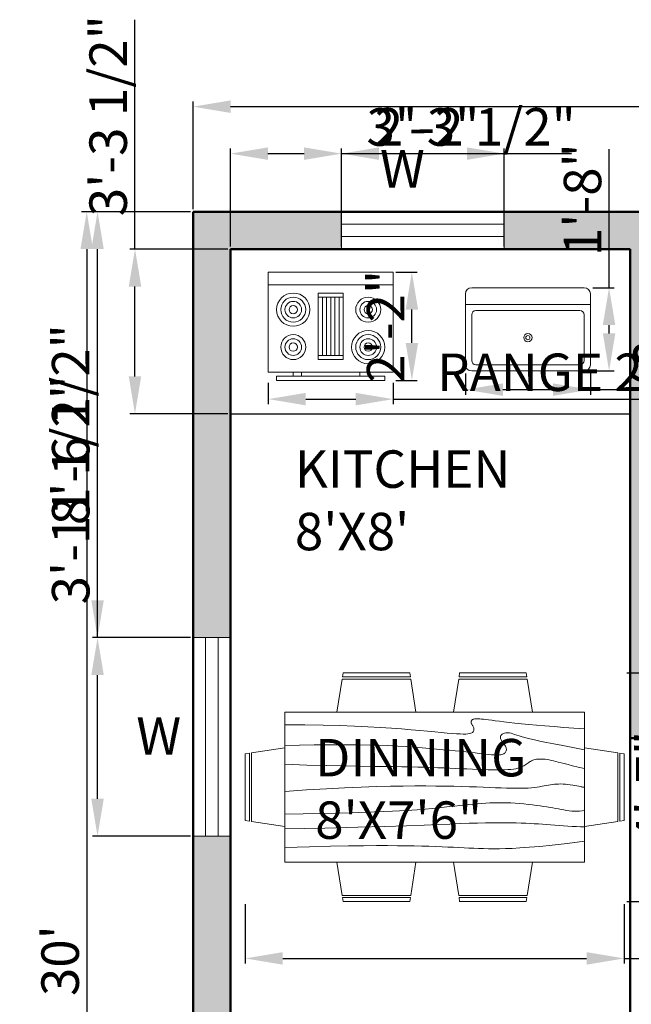
# Model space of a CAD drawing. Units: inches. Extents: x 16989 to 17950, y 7982 to 8536.
# Tile 2 of 5: x 16989 to 17136, y 8270 to 8506. Entities that reach past the tile are written whole.
import ezdxf

# ---------------------------------------------------------------- set-up
doc = ezdxf.new("R2010")
doc.units = ezdxf.units.IN
for name, color, linetype, lineweight in [('A-ANNO-DIMS', 2, 'Continuous', 18), ('A-ANNO-IDEN', 7, 'Continuous', 18), ('A-AREA-IDEN', 7, 'Continuous', 25), ('A-EQPM', 8, 'Continuous', 18), ('A-FLOR-CASE', 8, 'Continuous', 25), ('A-FLOR-FIXT', 9, 'Continuous', 18), ('A-FURN', 8, 'Continuous', 18), ('A-GLAZ', 4, 'Continuous', 18), ('A-WALL', 7, 'Continuous', 50)]:
    doc.layers.add(name, color=color, linetype=linetype, lineweight=lineweight)
doc.layers.add('A-WALL-PATT', color=177, linetype='Continuous', lineweight=13, true_color=0x293189)
doc.styles.get("Standard").update_dxf_attribs({"font": 'arial.ttf'})
doc.dimstyles.new('ISO-25', dxfattribs={"dimtxt": 9, "dimasz": 9, "dimexe": 1.25, "dimexo": 0.625, "dimtad": 1, "dimdec": 1, "dimrnd": 9, "dimlunit": 3, "dimtxsty": 'Standard', "dimcen": 2.5, "dimadec": 0, "dimazin": 0, "dimtfac": 1, "dimtdec": 1, "dimtmove": 0, "dimatfit": 3, "dimfxl": 1, "dimarcsym": 0})

# ---------------------------------------------------------------- blocks, each defined once
blk = doc.blocks.new('Range-Oven - 30 in top')
for p, q in [((0, -3), (30, -3)), ((12, -6), (18, -6)), ((13, -20), (13, -6)), ((14, -6), (14, -20)), ((15, -20), (15, -6)), ((16, -6), (16, -20)), ((17, -20), (17, -6)), ((18, -20), (12, -20)), ((6, -24), (6, -25)), ((8, -25), (8, -24)), ((22, -25), (22, -24)), ((24, -24), (24, -25))]:
    blk.add_line(p, q)
for points in [[(0, -24), (0, 0), (30, 0), (30, -24)], [(12, -21), (12, -5), (18, -5), (18, -21)], [(2, -26), (2, -25), (28, -25), (28, -26)]]:
    blk.add_lwpolyline(points, close=True)
for centre, radius in [((6, -9), 4), ((6, -9), 3), ((6, -9), 2), ((24, -9), 3), ((24, -9), 2), ((6, -9), 1), ((24, -9), 1), ((24, -18), 4), ((6, -18), 3), ((6, -18), 2), ((24, -18), 3), ((24, -18), 2), ((6, -18), 1), ((24, -18), 1)]:
    blk.add_circle(centre, radius)
blk = doc.blocks.new('Sink-single - 30 in top')
blk.add_line((-15, -3.999996), (15, -3.999996))
for points in [[(-13.5, 0), (13.5, 0)], [(-15, -18.499996), (-15, -1.5)], [(15, -1.5), (15, -18.499996)], [(-13.5, -17.499996), (-13.5, -6.499996)], [(-12.5, -5.499996), (12.5, -5.499996)], [(13.5, -6.499996), (13.5, -17.499996)], [(12.5, -18.499996), (-12.5, -18.499996)], [(13.5, -19.999996), (-13.5, -19.999996)]]:
    blk.add_lwpolyline(points)
for radius in [1, 0.5]:
    blk.add_circle((0, -11.999996), radius)
for centre, radius, start, end in [((-13.5, -1.5), 1.5, 90, 180), ((13.5, -1.5), 1.5, 0, 90), ((-12.5, -6.499996), 1, 90, 180), ((12.5, -6.499996), 1, 0, 90), ((-13.5, -18.499996), 1.5, 180, 270), ((-12.5, -17.499996), 1, 180, 270), ((12.5, -17.499996), 1, 270, 0), ((13.5, -18.499996), 1.5, 270, 0)]:
    blk.add_arc(centre, radius, start, end)
blk = doc.blocks.new('Dining Set - 36 x 72 in.')
for p, q in [((-22, 27.5), (-22.1562, 26.50042)), ((-5.8416, 26.5), (-22.1534, 26.5)), ((-22, 27.5), (-6, 27.5)), ((-5.8437, 26.49966), (-6, 27.5)), ((6, 27.5), (5.8438, 26.50042)), ((22.1584, 26.5), (5.8466, 26.5)), ((6, 27.5), (22, 27.5)), ((22.1563, 26.49966), (22, 27.5)), ((-22.2343, 26.00059), (-23.4847, 17.99762)), ((-22.2304, 26), (-5.7608, 26)), ((-4.5152, 17.99762), (-5.7655, 25.99926)), ((5.7657, 26.00059), (4.5153, 17.99762)), ((5.7696, 26), (22.2392, 26)), ((23.4848, 17.99762), (22.2345, 25.99926)), ((36, 18), (-36, 18)), ((-36, 18), (-36, -18)), ((36, -18), (36, 18)), ((-44.0006, 8.23428), (-35.9976, 9.48474)), ((44.0006, 8.23428), (35.9976, 9.48474)), ((-45.5, 8), (-44.5004, 8.15617)), ((-45.5, 8), (-45.5, -8)), ((-44.5, -8.15843), (-44.5, 8.15338)), ((-44, 8.23041), (-44, -8.23915)), ((44, 8.23041), (44, -8.23915)), ((44.5, -8.15843), (44.5, 8.15338)), ((45.5, 8), (44.5005, 8.15617)), ((45.5, 8), (45.5, -8)), ((-44.4997, -8.15631), (-45.5, -8)), ((-35.9976, -9.48476), (-43.9993, -8.2345)), ((35.9976, -9.48476), (43.9993, -8.2345)), ((44.4997, -8.15631), (45.5, -8)), ((-36, -18), (36, -18)), ((-22.2343, -26.0006), (-23.4847, -17.99762)), ((-4.5152, -17.99762), (-5.7655, -25.99928)), ((5.7657, -26.0006), (4.5153, -17.99762)), ((23.4848, -17.99762), (22.2345, -25.99928)), ((-22.2304, -26), (-5.7608, -26)), ((5.7696, -26), (22.2392, -26)), ((-22, -27.5), (-22.1562, -26.50044)), ((-5.8416, -26.5), (-22.1534, -26.5)), ((-22, -27.5), (-6, -27.5)), ((-5.8437, -26.49967), (-6, -27.5)), ((6, -27.5), (5.8438, -26.50044)), ((22.1584, -26.5), (5.8466, -26.5)), ((6, -27.5), (22, -27.5)), ((22.1563, -26.49967), (22, -27.5))]:
    blk.add_line(p, q)
for points in [[(-36, 15), (-31.1772, 14.97754), (-26.8079, 14.91406), (-22.8538, 14.81543), (-19.276, 14.6875), (-16.0362, 14.53613), (-13.0957, 14.36718), (-10.4159, 14.18652), (-7.9583, 14), (-5.6904, 13.81315), (-3.6035, 13.63021), (-1.6954, 13.45508), (0.0365, 13.29166), (1.5945, 13.14388), (2.9811, 13.01562), (4.1988, 12.9108), (5.25, 12.83333), (6.1393, 12.78613), (6.8802, 12.76823), (7.4883, 12.77767), (7.9792, 12.8125), (8.3685, 12.87077), (8.6719, 12.95052), (8.9049, 13.0498), (9.0833, 13.16666), (9.2205, 13.29899), (9.3216, 13.44401), (9.3895, 13.59879), (9.4271, 13.76041), (9.4373, 13.92594), (9.4232, 14.09245), (9.3875, 14.257), (9.3333, 14.41666), (9.2638, 14.56917), (9.1836, 14.71484), (9.0975, 14.85465), (9.0104, 14.98958), (8.9272, 15.1206), (8.8529, 15.2487), (8.7922, 15.37483), (8.75, 15.5), (8.7305, 15.62467), (8.7344, 15.74739), (8.7617, 15.86621), (8.8125, 15.97916), (8.8867, 16.08431), (8.9844, 16.17968), (9.1055, 16.26334), (9.25, 16.33333), (9.4189, 16.38802), (9.6172, 16.42708), (9.8506, 16.45052), (10.125, 16.45833), (10.4463, 16.45052), (10.8203, 16.42708), (11.2529, 16.38802), (11.75, 16.33333), (12.3184, 16.26318), (12.9694, 16.17838), (13.7151, 16.07991), (14.5677, 15.96875), (15.5395, 15.84586), (16.6426, 15.71224), (17.8893, 15.56884), (19.2917, 15.41666), (20.859, 15.25667), (22.5879, 15.08984), (24.4721, 14.91715), (26.5052, 14.73958), (28.6809, 14.5581), (30.9929, 14.3737), (33.4347, 14.18733), (36, 14)], [(-36, 10), (-28.9766, 10.14274), (-23.1725, 10.20442), (-18.4241, 10.19775), (-14.5677, 10.13541), (-11.4399, 10.03011), (-8.877, 9.89453), (-6.7154, 9.74137), (-4.7917, 9.58333), (-2.9698, 9.43082), (-1.2246, 9.28515), (0.4415, 9.14534), (2.026, 9.01041), (3.5266, 8.87939), (4.9408, 8.7513), (6.266, 8.62516), (7.5, 8.5), (8.6411, 8.37549), (9.6914, 8.2539), (10.6538, 8.13818), (11.5312, 8.03125), (12.3267, 7.93603), (13.043, 7.85547), (13.6831, 7.79248), (14.25, 7.75), (14.7471, 7.7303), (15.1797, 7.73307), (15.5537, 7.75732), (15.875, 7.80208), (16.1494, 7.86637), (16.3828, 7.94922), (16.5811, 8.04964), (16.75, 8.16666), (16.8944, 8.29915), (17.0143, 8.44531), (17.1089, 8.60319), (17.1771, 8.77083), (17.218, 8.94629), (17.2305, 9.1276), (17.2137, 9.31282), (17.1667, 9.5), (17.0895, 9.6875), (16.987, 9.875), (16.8649, 10.0625), (16.7292, 10.25), (16.5856, 10.4375), (16.4401, 10.625), (16.2985, 10.8125), (16.1667, 11), (16.05, 11.18733), (15.9518, 11.3737), (15.8752, 11.5581), (15.8229, 11.73958), (15.798, 11.91715), (15.8034, 12.08984), (15.842, 12.25667), (15.9167, 12.41666), (16.0295, 12.56836), (16.1784, 12.70833), (16.3605, 12.83268), (16.5729, 12.9375), (16.8127, 13.01888), (17.0768, 13.07291), (17.3625, 13.0957), (17.6667, 13.08333), (17.9894, 13.03312), (18.3418, 12.94726), (18.7382, 12.82918), (19.1927, 12.68229), (19.7195, 12.51001), (20.3327, 12.31575), (21.0465, 12.10294), (21.875, 11.875), (22.8357, 11.63354), (23.959, 11.37304), (25.2786, 11.08618), (26.8282, 10.76562), (28.6414, 10.40405), (30.752, 9.99414), (33.1936, 9.52856), (36, 9)], [(-36, 5.5), (-30.7157, 5.3348), (-26.069, 5.20963), (-21.9946, 5.11767), (-18.4271, 5.05208), (-15.3009, 5.00602), (-12.5508, 4.97265), (-10.1112, 4.94515), (-7.9167, 4.91666), (-5.909, 4.88167), (-4.0586, 4.83984), (-2.3429, 4.79215), (-0.7396, 4.73958), (0.7739, 4.6831), (2.22, 4.6237), (3.6213, 4.56233), (5, 4.5), (6.373, 4.43782), (7.7344, 4.3776), (9.0723, 4.32129), (10.375, 4.27083), (11.6309, 4.22819), (12.8281, 4.19531), (13.9551, 4.17415), (15, 4.16666), (15.954, 4.17448), (16.819, 4.19791), (17.6001, 4.23698), (18.3021, 4.29166), (18.9299, 4.36198), (19.4883, 4.44791), (19.9823, 4.54948), (20.4167, 4.66666), (20.7969, 4.79899), (21.1302, 4.94401), (21.4245, 5.09879), (21.6875, 5.26041), (21.9271, 5.42594), (22.1511, 5.59245), (22.3672, 5.757), (22.5834, 5.91666), (22.8065, 6.06868), (23.0404, 6.21093), (23.2879, 6.34147), (23.5521, 6.45833), (23.8358, 6.55957), (24.142, 6.64323), (24.4735, 6.70735), (24.8334, 6.75), (25.2235, 6.76969), (25.642, 6.76692), (26.0858, 6.74267), (26.5521, 6.69791), (27.0379, 6.63362), (27.5404, 6.55078), (28.0565, 6.45036), (28.5834, 6.33333), (29.1242, 6.19987), (29.7071, 6.04687), (30.3661, 5.87044), (31.1354, 5.66666), (32.0493, 5.43164), (33.142, 5.16146), (34.4475, 4.85221), (36, 4.5)], [(-36, -1), (-30.7915, -0.6591), (-26.0195, -0.38216), (-21.6519, -0.16284), (-17.6563, 0.00521), (-14.0005, 0.12833), (-10.6523, 0.21289), (-7.5796, 0.26522), (-4.75, 0.29166), (-2.134, 0.29793), (0.2878, 0.28711), (2.5317, 0.26163), (4.6146, 0.22396), (6.5529, 0.17651), (8.3633, 0.12174), (10.0623, 0.06209), (11.6667, 0), (13.1899, -0.06201), (14.6341, -0.1211), (15.9982, -0.17432), (17.2813, -0.21875), (18.4823, -0.25147), (19.6003, -0.26953), (20.6343, -0.27002), (21.5834, -0.25), (22.4481, -0.20768), (23.2357, -0.14584), (23.9549, -0.06836), (24.6146, 0.02083), (25.2235, 0.11784), (25.7904, 0.21875), (26.3241, 0.31966), (26.8334, 0.41666), (27.3265, 0.50618), (27.8099, 0.58593), (28.2894, 0.65397), (28.7709, 0.70833), (29.2601, 0.74707), (29.763, 0.76823), (30.2855, 0.76985), (30.8334, 0.75), (31.4088, 0.70784), (31.9994, 0.64713), (32.589, 0.57275), (33.1615, 0.48958), (33.7008, 0.4025), (34.1908, 0.3164), (34.6153, 0.23616), (34.9584, 0.16666), (35.2099, 0.11165), (35.3848, 0.07031), (35.504, 0.04069), (35.5886, 0.02083), (35.6594, 0.00879), (35.7377, 0.0026), (35.8442, 0.00032), (36, 0)], [(-36, -6.5), (-27.1843, -6.31267), (-20.084, -6.1263), (-14.469, -5.9419), (-10.1094, -5.76042), (-6.7752, -5.58285), (-4.2363, -5.41016), (-2.2629, -5.24333), (-0.625, -5.08334), (0.8708, -4.93099), (2.2715, -4.78646), (3.5872, -4.64974), (4.8281, -4.52084), (6.0046, -4.39974), (7.127, -4.28646), (8.2053, -4.18099), (9.25, -4.08334), (10.2705, -3.99382), (11.2734, -3.91407), (12.2647, -3.84603), (13.25, -3.79167), (14.2354, -3.75293), (15.2266, -3.73177), (16.2295, -3.73015), (17.25, -3.75), (18.2912, -3.79248), (19.3451, -3.85547), (20.4009, -3.93604), (21.4479, -4.03125), (22.4754, -4.13819), (23.4727, -4.25391), (24.4289, -4.37549), (25.3334, -4.5), (26.1785, -4.62492), (26.9694, -4.74935), (27.7145, -4.87281), (28.4219, -4.99479), (29.1, -5.11483), (29.7572, -5.23242), (30.4016, -5.34709), (31.0417, -5.45834), (31.6837, -5.56437), (32.3262, -5.65821), (32.9658, -5.73153), (33.599, -5.77604), (34.2224, -5.78345), (34.8327, -5.74545), (35.4264, -5.65373), (36, -5.5)], [(-36, -10), (-26.4022, -9.81299), (-18.4675, -9.62891), (-11.9839, -9.45069), (-6.7396, -9.28125), (-2.5226, -9.12354), (0.8789, -8.98047), (3.6769, -8.85498), (6.0833, -8.75), (8.2767, -8.66765), (10.3021, -8.60677), (12.1712, -8.56543), (13.8958, -8.54167), (15.4876, -8.53353), (16.9583, -8.53907), (18.3197, -8.55632), (19.5834, -8.58334), (20.7616, -8.61841), (21.8685, -8.66081), (22.9188, -8.71004), (23.9271, -8.76563), (24.9081, -8.82707), (25.8763, -8.89388), (26.8465, -8.96558), (27.8334, -9.04167), (28.8474, -9.12118), (29.8828, -9.20117), (30.93, -9.27824), (31.9792, -9.34896), (33.0205, -9.40991), (34.0443, -9.45768), (35.0407, -9.48885), (36, -9.5)], [(-36, -14.5), (-30.0881, -14.33513), (-25.0332, -14.21224), (-20.7312, -14.12647), (-17.0781, -14.07292), (-13.97, -14.04671), (-11.3027, -14.04297), (-8.9724, -14.05681), (-6.875, -14.08334), (-4.9224, -14.11833), (-3.0905, -14.16016), (-1.3709, -14.20785), (0.2448, -14.26042), (1.7647, -14.3169), (3.1973, -14.3763), (4.5507, -14.43767), (5.8333, -14.5), (7.0554, -14.5621), (8.235, -14.62175), (9.3922, -14.67652), (10.5469, -14.72396), (11.7192, -14.76164), (12.929, -14.78711), (14.1965, -14.79794), (15.5417, -14.79167), (16.9933, -14.76424), (18.6152, -14.70508), (20.4804, -14.60197), (22.6615, -14.44271), (25.2312, -14.21509), (28.2624, -13.9069), (31.8277, -13.50594), (36, -13)]]:
    blk.add_lwpolyline(points)
blk = doc.blocks.new('*D8')
at = {"layer": 'A-ANNO-DIMS', "color": 0, "lineweight": -2, "transparency": 16777216}
for p, q in [((17030.22, 8460.89), (17030.22, 8486.75)), ((17390.22, 8460.89), (17390.22, 8486.75)), ((17039.22, 8485.5), (17381.22, 8485.5))]:
    blk.add_line(p, q, dxfattribs=at)
at = {"layer": 'A-ANNO-DIMS', "color": 0, "transparency": 16777216}
for points in [[(17039.22, 8487), (17039.22, 8484), (17030.22, 8485.5)], [(17381.22, 8487), (17381.22, 8484), (17390.22, 8485.5)]]:
    blk.add_solid(points, dxfattribs=at)
at = {"layer": 'Defpoints', "color": 0, "transparency": 16777216}
for p in [(17390.22, 8485.5), (17030.22, 8460.26), (17390.22, 8460.26)]:
    blk.add_point(p, dxfattribs=at)
at = {"layer": 'A-ANNO-DIMS', "color": 0, "transparency": 16777216, "insert": (17210.22, 8490.72), "char_height": 9, "attachment_point": 5}
blk.add_mtext("30'", dxfattribs=at)
blk = doc.blocks.new('*D9')
at = {"layer": 'A-ANNO-DIMS', "color": 0, "lineweight": -2, "transparency": 16777216}
for p, q in [((17029.59, 8460.26), (17003.42, 8460.26)), ((17004.67, 8451.26), (17004.67, 8109.26)), ((17029.59, 8100.26), (17003.42, 8100.26))]:
    blk.add_line(p, q, dxfattribs=at)
at = {"layer": 'A-ANNO-DIMS', "color": 0, "transparency": 16777216}
for points in [[(17003.17, 8451.26), (17006.17, 8451.26), (17004.67, 8460.26)], [(17003.17, 8109.26), (17006.17, 8109.26), (17004.67, 8100.26)]]:
    blk.add_solid(points, dxfattribs=at)
at = {"layer": 'Defpoints', "color": 0, "transparency": 16777216}
for p in [(17030.22, 8460.26), (17004.67, 8100.26), (17030.22, 8100.26)]:
    blk.add_point(p, dxfattribs=at)
at = {"layer": 'A-ANNO-DIMS', "color": 0, "transparency": 16777216, "insert": (16999.45, 8280.26), "char_height": 9, "attachment_point": 5, "rotation": 90}
blk.add_mtext("30'", dxfattribs=at)
blk = doc.blocks.new('*D29')
at = {"layer": 'A-ANNO-DIMS', "color": 0, "lineweight": -2, "transparency": 16777216}
for p, q in [((17048.3, 8419.09), (17048.3, 8413.96)), ((17078.3, 8419.09), (17078.3, 8413.96)), ((17057.3, 8415.21), (17069.3, 8415.21)), ((17078.3, 8415.21), (17160.21, 8415.21))]:
    blk.add_line(p, q, dxfattribs=at)
at = {"layer": 'A-ANNO-DIMS', "color": 0, "transparency": 16777216}
for points in [[(17057.3, 8416.71), (17057.3, 8413.71), (17048.3, 8415.21)], [(17069.3, 8416.71), (17069.3, 8413.71), (17078.3, 8415.21)]]:
    blk.add_solid(points, dxfattribs=at)
at = {"layer": 'Defpoints', "color": 0, "transparency": 16777216}
for p in [(17048.3, 8419.71), (17078.3, 8419.71), (17078.3, 8415.21)]:
    blk.add_point(p, dxfattribs=at)
at = {"layer": 'A-ANNO-DIMS', "color": 0, "transparency": 16777216, "insert": (17123.75, 8420.49), "char_height": 9, "attachment_point": 5}
blk.add_mtext('RANGE 2\'-6"', dxfattribs=at)
blk = doc.blocks.new('*D30')
at = {"layer": 'A-ANNO-DIMS', "color": 0, "lineweight": -2, "transparency": 16777216}
for p, q in [((17078.92, 8445.71), (17084.05, 8445.71)), ((17082.8, 8428.71), (17082.8, 8436.71)), ((17078.92, 8419.71), (17084.05, 8419.71))]:
    blk.add_line(p, q, dxfattribs=at)
at = {"layer": 'A-ANNO-DIMS', "color": 0, "transparency": 16777216}
for points in [[(17081.3, 8436.71), (17084.3, 8436.71), (17082.8, 8445.71)], [(17081.3, 8428.71), (17084.3, 8428.71), (17082.8, 8419.71)]]:
    blk.add_solid(points, dxfattribs=at)
at = {"layer": 'Defpoints', "color": 0, "transparency": 16777216}
for p in [(17078.3, 8445.71), (17082.8, 8445.71), (17078.3, 8419.71)]:
    blk.add_point(p, dxfattribs=at)
at = {"layer": 'A-ANNO-DIMS', "color": 0, "transparency": 16777216, "insert": (17077.66, 8432.71), "char_height": 9, "attachment_point": 5, "rotation": 90}
blk.add_mtext('2\'-2"', dxfattribs=at)
blk = doc.blocks.new('*D31')
at = {"layer": 'A-ANNO-DIMS', "color": 0, "lineweight": -2, "transparency": 16777216}
for p, q in [((17095.68, 8421.36), (17095.68, 8416.24)), ((17125.68, 8421.36), (17125.68, 8416.24)), ((17104.68, 8417.49), (17116.68, 8417.49)), ((17125.68, 8417.49), (17192.65, 8417.49))]:
    blk.add_line(p, q, dxfattribs=at)
at = {"layer": 'A-ANNO-DIMS', "color": 0, "transparency": 16777216}
for points in [[(17104.68, 8418.99), (17104.68, 8415.99), (17095.68, 8417.49)], [(17116.68, 8418.99), (17116.68, 8415.99), (17125.68, 8417.49)]]:
    blk.add_solid(points, dxfattribs=at)
at = {"layer": 'Defpoints', "color": 0, "transparency": 16777216}
for p in [(17095.68, 8421.99), (17125.68, 8421.99), (17125.68, 8417.49)]:
    blk.add_point(p, dxfattribs=at)
at = {"layer": 'A-ANNO-DIMS', "color": 0, "transparency": 16777216, "insert": (17163.66, 8422.77), "char_height": 9, "attachment_point": 5}
blk.add_mtext('SINK 2\'-6"', dxfattribs=at)
blk = doc.blocks.new('*D32')
at = {"layer": 'A-ANNO-DIMS', "color": 0, "lineweight": -2, "transparency": 16777216}
for p, q in [((17130.18, 8441.99), (17130.18, 8475.32)), ((17126.3, 8441.99), (17131.43, 8441.99)), ((17130.18, 8430.99), (17130.18, 8432.99)), ((17126.3, 8421.99), (17131.43, 8421.99))]:
    blk.add_line(p, q, dxfattribs=at)
at = {"layer": 'A-ANNO-DIMS', "color": 0, "transparency": 16777216}
for points in [[(17128.68, 8432.99), (17131.68, 8432.99), (17130.18, 8441.99)], [(17128.68, 8430.99), (17131.68, 8430.99), (17130.18, 8421.99)]]:
    blk.add_solid(points, dxfattribs=at)
at = {"layer": 'Defpoints', "color": 0, "transparency": 16777216}
for p in [(17125.68, 8441.99), (17130.18, 8441.99), (17125.68, 8421.99)]:
    blk.add_point(p, dxfattribs=at)
at = {"layer": 'A-ANNO-DIMS', "color": 0, "transparency": 16777216, "insert": (17124.96, 8463.15), "char_height": 9, "attachment_point": 5, "rotation": 90}
blk.add_mtext('1\'-8"', dxfattribs=at)
blk = doc.blocks.new('*D33')
at = {"layer": 'A-ANNO-DIMS', "color": 0, "lineweight": -2, "transparency": 16777216}
for p, q in [((17042.78, 8293.82), (17042.78, 8279.54)), ((17133.78, 8293.82), (17133.78, 8279.54)), ((17051.78, 8280.79), (17124.78, 8280.79)), ((17133.78, 8280.79), (17242.95, 8280.79))]:
    blk.add_line(p, q, dxfattribs=at)
at = {"layer": 'A-ANNO-DIMS', "color": 0, "transparency": 16777216}
for points in [[(17051.78, 8282.29), (17051.78, 8279.29), (17042.78, 8280.79)], [(17124.78, 8282.29), (17124.78, 8279.29), (17133.78, 8280.79)]]:
    blk.add_solid(points, dxfattribs=at)
at = {"layer": 'Defpoints', "color": 0, "transparency": 16777216}
for p in [(17042.78, 8294.44), (17133.78, 8294.44), (17133.78, 8280.79)]:
    blk.add_point(p, dxfattribs=at)
at = {"layer": 'A-ANNO-DIMS', "color": 0, "transparency": 16777216, "insert": (17192.87, 8286.07), "char_height": 9, "attachment_point": 5}
blk.add_mtext('DINING SET 7\'-7"', dxfattribs=at)
blk = doc.blocks.new('*D34')
at = {"layer": 'A-ANNO-DIMS', "color": 0, "lineweight": -2, "transparency": 16777216}
for p, q in [((17134.41, 8349.44), (17148.68, 8349.44)), ((17147.43, 8303.44), (17147.43, 8340.44)), ((17134.41, 8294.44), (17148.68, 8294.44))]:
    blk.add_line(p, q, dxfattribs=at)
at = {"layer": 'A-ANNO-DIMS', "color": 0, "transparency": 16777216}
for points in [[(17145.93, 8340.44), (17148.93, 8340.44), (17147.43, 8349.44)], [(17145.93, 8303.44), (17148.93, 8303.44), (17147.43, 8294.44)]]:
    blk.add_solid(points, dxfattribs=at)
at = {"layer": 'Defpoints', "color": 0, "transparency": 16777216}
for p in [(17133.78, 8349.44), (17147.43, 8349.44), (17133.78, 8294.44)]:
    blk.add_point(p, dxfattribs=at)
at = {"layer": 'A-ANNO-DIMS', "color": 0, "transparency": 16777216, "insert": (17142.31, 8321.94), "char_height": 9, "attachment_point": 5, "rotation": 90}
blk.add_mtext('4\'-7"', dxfattribs=at)
blk = doc.blocks.new('*D35')
at = {"layer": 'A-ANNO-DIMS', "color": 0, "lineweight": -2, "transparency": 16777216}
for p, q in [((17039.22, 8451.89), (17039.22, 8475.46)), ((17048.22, 8474.21), (17056.89, 8474.21)), ((17065.89, 8451.89), (17065.89, 8475.46)), ((17065.89, 8474.21), (17121.19, 8474.21))]:
    blk.add_line(p, q, dxfattribs=at)
at = {"layer": 'A-ANNO-DIMS', "color": 0, "transparency": 16777216}
for points in [[(17048.22, 8475.71), (17048.22, 8472.71), (17039.22, 8474.21)], [(17056.89, 8475.71), (17056.89, 8472.71), (17065.89, 8474.21)]]:
    blk.add_solid(points, dxfattribs=at)
at = {"layer": 'Defpoints', "color": 0, "transparency": 16777216}
for p in [(17065.89, 8474.21), (17039.22, 8451.26), (17065.89, 8451.26)]:
    blk.add_point(p, dxfattribs=at)
at = {"layer": 'A-ANNO-DIMS', "color": 0, "transparency": 16777216, "insert": (17098.04, 8479.49), "char_height": 9, "attachment_point": 5}
blk.add_mtext('2\'-2 1/2"', dxfattribs=at)
blk = doc.blocks.new('*D36')
at = {"layer": 'A-ANNO-DIMS', "color": 0, "lineweight": -2, "transparency": 16777216}
for p, q in [((17065.89, 8451.89), (17065.89, 8475.46)), ((17074.89, 8474.21), (17096.01, 8474.21)), ((17105.01, 8451.89), (17105.01, 8475.46))]:
    blk.add_line(p, q, dxfattribs=at)
at = {"layer": 'A-ANNO-DIMS', "color": 0, "transparency": 16777216}
for points in [[(17074.89, 8475.71), (17074.89, 8472.71), (17065.89, 8474.21)], [(17096.01, 8475.71), (17096.01, 8472.71), (17105.01, 8474.21)]]:
    blk.add_solid(points, dxfattribs=at)
at = {"layer": 'Defpoints', "color": 0, "transparency": 16777216}
for p in [(17105.01, 8474.21), (17065.89, 8451.26), (17105.01, 8451.26)]:
    blk.add_point(p, dxfattribs=at)
at = {"layer": 'A-ANNO-DIMS', "color": 0, "transparency": 16777216, "insert": (17085.45, 8479.43), "char_height": 9, "attachment_point": 5}
blk.add_mtext('3\'-3"', dxfattribs=at)
blk = doc.blocks.new('*D45')
at = {"layer": 'A-ANNO-DIMS', "color": 0, "lineweight": -2, "transparency": 16777216}
for p, q in [((17029.59, 8460.26), (17006.02, 8460.26)), ((17007.27, 8366.88), (17007.27, 8451.26)), ((17029.59, 8357.88), (17006.02, 8357.88))]:
    blk.add_line(p, q, dxfattribs=at)
at = {"layer": 'A-ANNO-DIMS', "color": 0, "transparency": 16777216}
for points in [[(17005.77, 8451.26), (17008.77, 8451.26), (17007.27, 8460.26)], [(17005.77, 8366.88), (17008.77, 8366.88), (17007.27, 8357.88)]]:
    blk.add_solid(points, dxfattribs=at)
at = {"layer": 'Defpoints', "color": 0, "transparency": 16777216}
for p in [(17007.27, 8460.26), (17030.22, 8460.26), (17030.22, 8357.88)]:
    blk.add_point(p, dxfattribs=at)
at = {"layer": 'A-ANNO-DIMS', "color": 0, "transparency": 16777216, "insert": (17001.99, 8409.07), "char_height": 9, "attachment_point": 5, "rotation": 90}
blk.add_mtext('8\'-6 1/2"', dxfattribs=at)
blk = doc.blocks.new('*D46')
at = {"layer": 'A-ANNO-DIMS', "color": 0, "lineweight": -2, "transparency": 16777216}
for p, q in [((17007.27, 8357.88), (17007.27, 8420.02)), ((17029.59, 8357.88), (17006.02, 8357.88)), ((17007.27, 8319.16), (17007.27, 8348.88)), ((17029.59, 8310.16), (17006.02, 8310.16))]:
    blk.add_line(p, q, dxfattribs=at)
at = {"layer": 'A-ANNO-DIMS', "color": 0, "transparency": 16777216}
for points in [[(17005.77, 8348.88), (17008.77, 8348.88), (17007.27, 8357.88)], [(17005.77, 8319.16), (17008.77, 8319.16), (17007.27, 8310.16)]]:
    blk.add_solid(points, dxfattribs=at)
at = {"layer": 'Defpoints', "color": 0, "transparency": 16777216}
for p in [(17007.27, 8357.88), (17030.22, 8357.88), (17030.22, 8310.16)]:
    blk.add_point(p, dxfattribs=at)
at = {"layer": 'A-ANNO-DIMS', "color": 0, "transparency": 16777216, "insert": (17001.99, 8393.45), "char_height": 9, "attachment_point": 5, "rotation": 90}
blk.add_mtext('3\'-11 1/2"', dxfattribs=at)
blk = doc.blocks.new('*D66')
at = {"layer": 'A-ANNO-DIMS', "color": 0, "lineweight": -2, "transparency": 16777216}
for p, q in [((17016.27, 8451.26), (17016.27, 8506.4)), ((17038.59, 8451.26), (17015.02, 8451.26)), ((17016.27, 8420.68), (17016.27, 8442.26)), ((17038.59, 8411.68), (17015.02, 8411.68))]:
    blk.add_line(p, q, dxfattribs=at)
at = {"layer": 'A-ANNO-DIMS', "color": 0, "transparency": 16777216}
for points in [[(17014.77, 8442.26), (17017.77, 8442.26), (17016.27, 8451.26)], [(17014.77, 8420.68), (17017.77, 8420.68), (17016.27, 8411.68)]]:
    blk.add_solid(points, dxfattribs=at)
at = {"layer": 'Defpoints', "color": 0, "transparency": 16777216}
for p in [(17016.27, 8451.26), (17039.22, 8451.26), (17039.22, 8411.68)]:
    blk.add_point(p, dxfattribs=at)
at = {"layer": 'A-ANNO-DIMS', "color": 0, "transparency": 16777216, "insert": (17010.99, 8483.33), "char_height": 9, "attachment_point": 5, "rotation": 90}
blk.add_mtext('3\'-3 1/2"', dxfattribs=at)

msp = doc.modelspace()

# ---------------------------------------------------------------- hatches: boundary and pattern name
at = {"layer": 'A-WALL-PATT'}
h = msp.add_hatch(color=256, dxfattribs=at)
h.dxf.hatch_style = 1
h.paths.add_polyline_path([(17039.22, 8310.16), (17030.22, 8310.16), (17030.22, 8100.26), (17049.62, 8100.26), (17049.62, 8109.26), (17039.22, 8109.26), (17039.22, 8256.26), (17144.22, 8256.26), (17144.22, 8265.26), (17039.22, 8265.26)])
h.paths.add_polyline_path([(17039.22, 8451.26), (17065.89, 8451.26), (17065.89, 8460.26), (17030.22, 8460.26), (17030.22, 8357.88), (17039.22, 8357.88)])
h.paths.add_polyline_path([(17180.39, 8460.26), (17105.01, 8460.26), (17105.01, 8451.26), (17135.22, 8451.26), (17135.22, 8333.76), (17144.22, 8333.76), (17144.22, 8451.26), (17180.39, 8451.26)])
h.paths.add_polyline_path([(17309.67, 8460.26), (17217.66, 8460.26), (17217.66, 8451.26), (17258.22, 8451.26), (17258.22, 8304.98), (17262.72, 8304.98, -0.013209), (17264.26, 8304.98), (17267.22, 8304.98), (17267.22, 8394.26), (17348.26, 8394.26), (17348.26, 8403.26), (17267.22, 8403.26), (17267.22, 8451.26), (17309.67, 8451.26)])
h.paths.add_polyline_path([(17390.22, 8460.26), (17336.17, 8460.26), (17336.17, 8451.26), (17381.22, 8451.26), (17381.22, 8403.26), (17381.22, 8394.26), (17381.22, 8367.17), (17390.22, 8367.17)])
h.paths.add_polyline_path([(17390.22, 8325.05), (17381.22, 8325.05), (17381.22, 8274.26), (17267.22, 8274.26), (17258.22, 8274.26), (17258.22, 8265.26), (17267.22, 8265.26), (17381.22, 8265.26), (17381.22, 8238), (17390.22, 8238)])
h.paths.add_polyline_path([(17390.22, 8194.87), (17381.22, 8194.87), (17381.22, 8157.26), (17381.22, 8148.26), (17381.22, 8109.26), (17332.58, 8109.26), (17332.58, 8100.26), (17390.22, 8100.26)])
h.paths.add_polyline_path([(17349.64, 8157.26), (17267.22, 8157.26), (17267.22, 8231.5), (17258.22, 8231.5), (17258.22, 8193.26), (17144.22, 8193.26), (17114.21, 8193.26), (17114.21, 8184.26), (17144.22, 8184.26), (17258.22, 8184.26), (17258.22, 8109.26), (17088.6, 8109.26), (17088.6, 8100.26), (17308.63, 8100.26), (17308.63, 8109.26), (17267.22, 8109.26), (17267.22, 8148.26), (17349.64, 8148.26)])

# ---------------------------------------------------------------- linework, layer by layer
at = {"layer": 'A-FLOR-CASE'}
msp.add_line((17039.22, 8411.68), (17135.22, 8411.68), dxfattribs=at)
at = {"layer": 'A-GLAZ'}
for p, q in [((17065.89, 8460.26), (17065.89, 8451.26)), ((17105.01, 8460.26), (17105.01, 8451.26)), ((17105.01, 8457.26), (17065.89, 8457.26)), ((17105.01, 8454.26), (17065.89, 8454.26)), ((17039.22, 8357.88), (17030.22, 8357.88)), ((17033.22, 8357.88), (17033.22, 8310.16)), ((17036.22, 8357.88), (17036.22, 8310.16)), ((17039.22, 8310.16), (17030.22, 8310.16))]:
    msp.add_line(p, q, dxfattribs=at)
at = {"layer": 'A-WALL'}
for p, q in [((17390.22, 8460.26), (17030.22, 8460.26)), ((17030.22, 8460.26), (17030.22, 8100.26)), ((17039.22, 8451.26), (17039.22, 8265.26)), ((17135.22, 8451.26), (17039.22, 8451.26)), ((17135.22, 8451.26), (17135.22, 8265.26)), ((17144.22, 8333.76), (17135.22, 8333.76))]:
    msp.add_line(p, q, dxfattribs=at)

# ---------------------------------------------------------------- block references
at = {"layer": 'A-EQPM'}
msp.add_blockref('Range-Oven - 30 in top', (17048.3, 8445.71), dxfattribs=at)
at = {"layer": 'A-FLOR-FIXT'}
msp.add_blockref('Sink-single - 30 in top', (17110.68, 8441.99), dxfattribs=at)
at = {"layer": 'A-FURN'}
msp.add_blockref('Dining Set - 36 x 72 in.', (17088.28, 8321.94), dxfattribs=at)

# ---------------------------------------------------------------- texts
at = {"layer": 'A-ANNO-IDEN', "char_height": 9, "attachment_point": 1}
for insert in [(17075.13, 8475.05), (17016.58, 8338.73)]:
    msp.add_mtext_dynamic_manual_height_columns('W', width=19.3379, gutter_width=12.5, heights=[0], dxfattribs=dict(at, insert=insert))
at = {"layer": 'A-AREA-IDEN', "char_height": 9, "attachment_point": 1}
for s, insert in [("KITCHEN\\P8'X8'", (17054.69, 8402.89)), ('DINNING\\P8\'X7\'6"', (17059.57, 8333.53))]:
    msp.add_mtext_dynamic_manual_height_columns(s, width=65.8099, gutter_width=12.5, heights=[0], dxfattribs=dict(at, insert=insert))

# ---------------------------------------------------------------- dimensions: what is measured, and where the dimension line sits
at = {"layer": 'A-ANNO-DIMS'}
for base, p1, p2, override, picture, middle in [((17016.27, 8451.26), (17039.22, 8411.68), (17039.22, 8451.26), {"dimdec": 1, "dimlfac": 1, "dimrnd": 0, "dimzin": 1, "dimdsep": 46, "dimlunit": 4, "dimfrac": 2}, '*D66', (17010.99, 8483.33)), ((17130.18, 8441.99), (17125.68, 8421.99), (17125.68, 8441.99), {"dimdec": 1, "dimlfac": 1, "dimrnd": 0, "dimzin": 1, "dimdsep": 46, "dimlunit": 4, "dimfrac": 2}, '*D32', (17124.96, 8463.15)), ((17007.27, 8460.26), (17030.22, 8357.88), (17030.22, 8460.26), {"dimdec": 1, "dimlfac": 1, "dimrnd": 0, "dimzin": 1, "dimdsep": 46, "dimlunit": 4, "dimfrac": 2}, '*D45', (17001.99, 8409.07)), ((17004.67, 8100.26), (17030.22, 8460.26), (17030.22, 8100.26), {"dimclrd": 0, "dimclre": 0, "dimclrt": 0}, '*D9', (16999.45, 8280.26)), ((17082.8, 8445.71), (17078.3, 8419.71), (17078.3, 8445.71), {"dimdec": 1, "dimlfac": 1, "dimrnd": 0, "dimzin": 1, "dimdsep": 46, "dimlunit": 4, "dimfrac": 2}, '*D30', (17077.66, 8432.71)), ((17007.27, 8357.88), (17030.22, 8310.16), (17030.22, 8357.88), {"dimdec": 1, "dimlfac": 1, "dimrnd": 0, "dimzin": 1, "dimdsep": 46, "dimlunit": 4, "dimfrac": 2}, '*D46', (17001.99, 8393.45)), ((17147.43, 8349.44), (17133.78, 8294.44), (17133.78, 8349.44), {"dimdec": 1, "dimlfac": 1, "dimrnd": 0, "dimzin": 1, "dimdsep": 46, "dimlunit": 4, "dimfrac": 2}, '*D34', (17142.31, 8321.94))]:
    dim = msp.add_linear_dim(base=base, p1=p1, p2=p2, angle=90, dimstyle='ISO-25', override=override, dxfattribs=at)
    dim.commit()
    dim.dimension.update_dxf_attribs({"geometry": picture, "text_midpoint": middle})
for base, p1, p2, override, picture, middle in [((17390.22, 8485.5), (17030.22, 8460.26), (17390.22, 8460.26), {"dimclrd": 0, "dimclre": 0, "dimclrt": 0}, '*D8', (17210.22, 8490.72)), ((17065.89, 8474.21), (17039.22, 8451.26), (17065.89, 8451.26), {"dimdec": 1, "dimlfac": 1, "dimrnd": 0, "dimzin": 1, "dimdsep": 46, "dimlunit": 4, "dimfrac": 2}, '*D35', (17098.04, 8479.49)), ((17105.01, 8474.21), (17065.89, 8451.26), (17105.01, 8451.26), {"dimdec": 1, "dimlfac": 1, "dimrnd": 0, "dimzin": 1, "dimdsep": 46, "dimlunit": 4, "dimfrac": 2}, '*D36', (17085.45, 8479.43))]:
    dim = msp.add_linear_dim(base=base, p1=p1, p2=p2, dimstyle='ISO-25', override=override, dxfattribs=at)
    dim.commit()
    dim.dimension.update_dxf_attribs({"geometry": picture, "text_midpoint": middle})
for base, p1, p2, text, picture, middle in [((17078.3, 8415.21), (17048.3, 8419.71), (17078.3, 8419.71), 'RANGE <>', '*D29', (17123.75, 8420.49)), ((17125.68, 8417.49), (17095.68, 8421.99), (17125.68, 8421.99), 'SINK <>', '*D31', (17163.66, 8422.77)), ((17133.78, 8280.79), (17042.78, 8294.44), (17133.78, 8294.44), 'DINING SET <>', '*D33', (17192.87, 8286.07))]:
    dim = msp.add_linear_dim(base=base, p1=p1, p2=p2, text=text, dimstyle='ISO-25', override={"dimdec": 1, "dimlfac": 1, "dimrnd": 0, "dimzin": 1, "dimdsep": 46, "dimlunit": 4, "dimfrac": 2}, dxfattribs=at)
    dim.commit()
    dim.dimension.update_dxf_attribs({"geometry": picture, "text_midpoint": middle})

doc.saveas('drawing.dxf')
